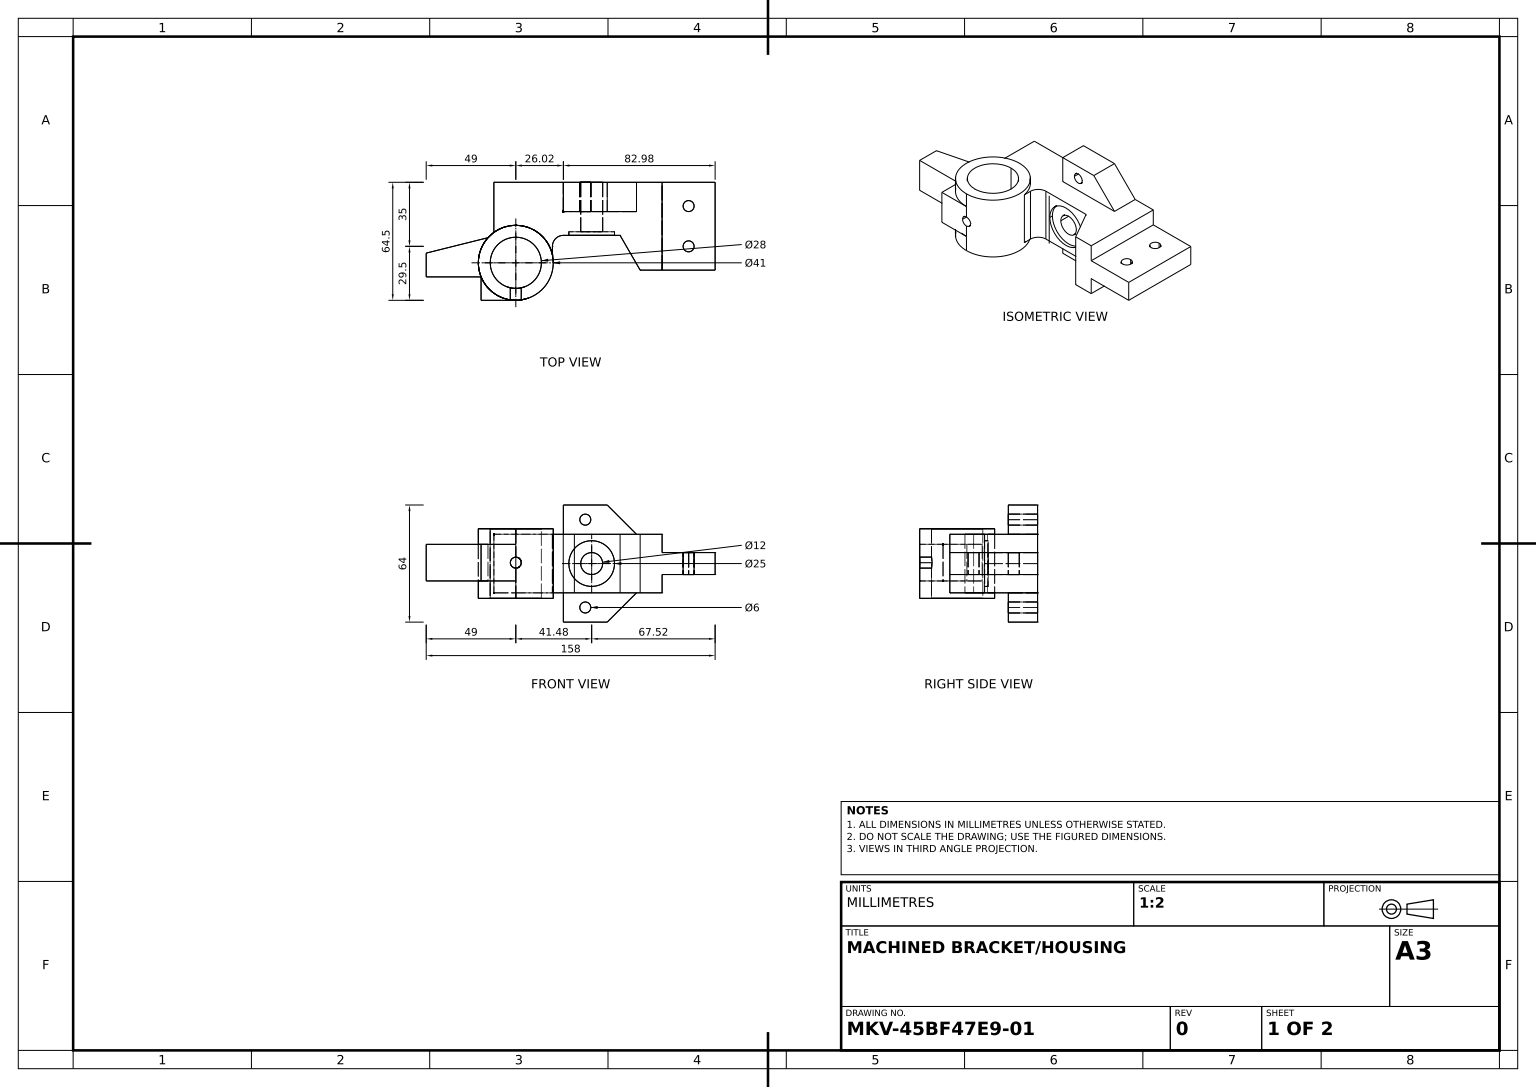
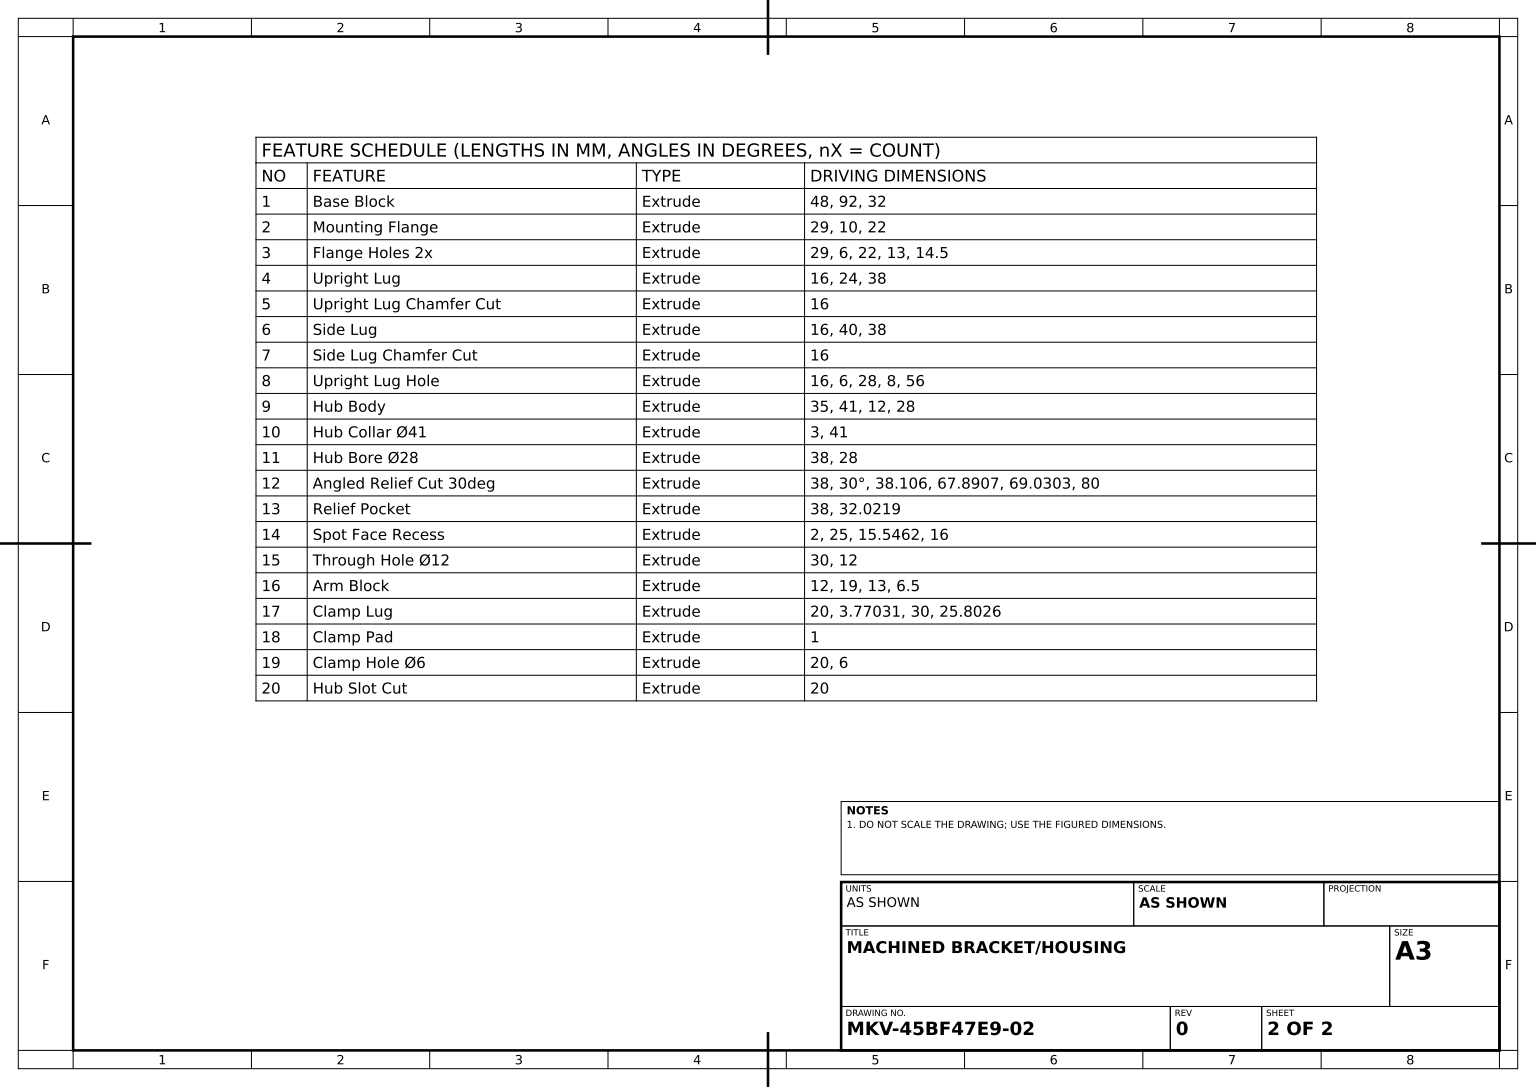
SolidWorks part; units mm, degrees
material "Plain Carbon Steel"
ref_plane "Front Plane" through (0, 0, 0) normal (0, 0, 1) x (1, 0, 0)
ref_plane "Top Plane" through (0, 0, 0) normal (0, 1, 0) x (1, 0, 0)
ref_plane "Right Plane" through (0, 0, 0) normal (1, 0, 0) x (0, 0, -1)
sketch "Base Block Sketch" plane through (0, 0, 0) normal (0, 0, 1) x (1, 0, 0)
  line L0 (0, 0) -> (92, 0)
  line L1 (92, 0) -> (92, 32)
  line L2 (92, 32) -> (0, 32)
  line L3 (0, 32) -> (0, 0)
  dimension "D1" = 92
  dimension "D2" = 32
extrude "Base Block" add sketch "Base Block Sketch" along normal blind 48
sketch "Mounting Flange Sketch" plane through (92, 0, 0) normal (1, 0, 0) x (0, 0, -1)
  line L0 (-48, 22) -> (-48, 10)
  line L1 (-48, 0) -> (-48, 32) construction
  line L2 (-48, 22) -> (0, 22)
  line L3 (0, 0) -> (0, 32) construction
  line L4 (0, 22) -> (0, 10)
  line L5 (0, 10) -> (-48, 10)
  line L6 (-48, 32) -> (0, 32) construction
  dimension "D1" = 10
  dimension "D2" = 22
extrude "Mounting Flange" add sketch "Mounting Flange Sketch" along normal blind 29
sketch "Flange Holes Sketch" plane through (0, 10, 0) normal (0, -1, 0) x (1, 0, 0)
  line L0 (121, 0) -> (92, 0) construction
  line L2 (121, 48) -> (121, 0) construction
  circle A0 centre (106.5, 13) radius 3
  circle A1 centre (106.5, 35) radius 3
  dimension "D1" = 6
  dimension "D2" = 6
  dimension "D3" = 22
  dimension "D4" = 13
  dimension "D5" = 14.5
  dimension "D6" = 14.5
extrude "Flange Holes 2x" cut sketch "Flange Holes Sketch" against normal blind 29
sketch "Upright Lug Sketch" plane through (0, 0, 0) normal (0, -1, 0) x (1, 0, 0)
  line L1 (0, 0) -> (92, 0) construction
  line L2 (38, 0) -> (62, 0)
  line L3 (62, 0) -> (78, 0)
  line L4 (78, 0) -> (78, 16)
  line L5 (78, 16) -> (62, 16)
  line L6 (62, 16) -> (38, 16)
  line L7 (38, 16) -> (38, 0)
  dimension "D1" = 16
  dimension "D2" = 24
  dimension "D3" = 16
  dimension "D4" = 16
  dimension "D5" = 38
extrude "Upright Lug" add sketch "Upright Lug Sketch" along normal blind 16
sketch "Upright Lug Chamfer Sketch" plane through (0, 0, 16) normal (0, 0, 1) x (1, 0, 0)
  line L0 (78, -16) -> (62, -16)
  line L1 (78, -16) -> (38, -16) construction
  line L2 (62, -16) -> (78, 0)
  line L3 (78, 0) -> (78, -16)
extrude "Upright Lug Chamfer Cut" cut sketch "Upright Lug Chamfer Sketch" against normal blind 16
sketch "Side Lug Sketch" plane through (0, 32, 0) normal (0, 1, 0) x (1, 0, 0)
  line L0 (0, -48) -> (0, 0) construction
  line L1 (92, 0) -> (0, 0) construction
  line L2 (38, 0) -> (62, 0)
  line L3 (62, 0) -> (78, 0)
  line L4 (78, 0) -> (78, -16)
  line L5 (78, -16) -> (62, -16)
  line L6 (62, -16) -> (38, -16)
  line L7 (38, -16) -> (38, 0)
  dimension "D1" = 16
  dimension "D2" = 40
  dimension "D3" = 38
extrude "Side Lug" add sketch "Side Lug Sketch" along normal blind 16
sketch "Side Lug Chamfer Sketch" plane through (0, 0, 16) normal (0, 0, 1) x (1, 0, 0)
  line L0 (78, 48) -> (62, 48)
  line L1 (38, 48) -> (78, 48) construction
  line L2 (62, 48) -> (78, 32)
  line L3 (78, 32) -> (78, 48)
extrude "Side Lug Chamfer Cut" cut sketch "Side Lug Chamfer Sketch" against normal blind 16
sketch "Upright Lug Hole Sketch" plane through (0, 0, 16) normal (0, 0, 1) x (1, 0, 0)
  line L0 (62, -16) -> (38, -16) construction
  circle A0 centre (50, 40) radius 3
  circle A1 centre (50, -8) radius 3
  dimension "D1" = 6
  dimension "D2" = 6
  dimension "D3" = 6
  dimension "D4" = 6
  dimension "D5" = 28
  dimension "D6" = 8
  dimension "D7" = 56
extrude "Upright Lug Hole" cut sketch "Upright Lug Hole Sketch" against normal blind 16
sketch "Hub Body Sketch" plane through (0, 0, 0) normal (0, -1, 0) x (1, 0, 0)
  line L0 (0, 0) -> (12, 0)
  line L1 (0, 0) -> (38, 0) construction
  line L2 (0, 48) -> (0, 0) construction
  line L4 (78, 16) -> (38, 16) construction
  circle A0 centre (12, 44) radius 20.5
  line M6 (92, 48) -> (0, 48)
  line M7 (0, 48) -> (0, 0)
  dimension "D1" = 41
  dimension "D2" = 41
  dimension "D3" = 12
  dimension "D4" = 28
extrude "Hub Body" add sketch "Hub Body Sketch" against normal blind 35 contours A0 M6 M7 | A0 M7 M6
sketch "Hub Collar Sketch" plane through (0, 0, 0) normal (0, -1, 0) x (1, 0, 0)
  circle A0 centre (12, 44) radius 20.5
  dimension "D1" = 41
  dimension "D2" = 41
extrude "Hub Collar Ø41" add sketch "Hub Collar Sketch" along normal blind 3
sketch "Hub Bore Sketch" plane through (0, -3, 0) normal (0, -1, 0) x (1, 0, 0)
  circle A0 centre (12, 44) radius 14
  dimension "D1" = 28
  dimension "D2" = 28
extrude "Hub Bore Ø28" cut sketch "Hub Bore Sketch" against normal blind 38
sketch "Angled Relief Sketch" plane through (0, 0, 0) normal (0, -1, 0) x (1, 0, 0)
  line L0 (92, 48) -> (80, 48)
  line L1 (32.106, 48) -> (92, 48) construction
  line L2 (80, 48) -> (69.0303, 29)
  line L3 (0, 27.3792) -> (0, 0) construction
  line L4 (67.8907, 29) -> (69.0303, 29)
  line L6 (92, 48) -> (92, 0) construction
  line L8 (67.8907, 29) -> (38.106, 29)
  line L10 (38.106, 48) -> (80, 48)
  line L11 (38.106, 48) -> (38.106, 29)
  line L12 (38.106, 48) -> (80, 48)
  point P11 (32.106, 48)
  line M11 (92, 48) -> (32.106, 48)
  dimension "D2" = 38.106
  dimension "D1" = 30
  dimension "D3" = 67.8907
  dimension "D4" = 69.0303
  dimension "D5" = 80
extrude "Angled Relief Cut 30deg" cut sketch "Angled Relief Sketch" against normal blind 38 contours L11 L8 L4 L2 M11
sketch "Relief Pocket Sketch" plane through (0, 0, 0) normal (0, -1, 0) x (1, 0, 0)
  line L0 (32.0219, 34.9994) -> (32.106, 48)
  line L1 (0, 27.3792) -> (0, 0) construction
  line L2 (38.106, 29) -> (37.9379, 29)
  line L5 (32.106, 48) -> (38.106, 48)
  line L6 (38.106, 48) -> (38.106, 29)
  arc A0 (32.0219, 34.9994) -> (38.106, 29) centre (38.0219, 34.9994) ccw
  line M3 (38.106, 29) -> (38.106, 48)
  line M4 (38.106, 48) -> (32.106, 48)
  arc M5 (32.106, 48) -> (0, 27.3792) centre (12, 44) cw
  dimension "D1" = 6
  dimension "D2" = 32.0219
extrude "Relief Pocket" cut sketch "Relief Pocket Sketch" against normal blind 38 contours L0 A0 L2 M3 M4 M5
sketch "Spot Face Sketch" plane through (0, 0, 29) normal (0, 0, 1) x (1, 0, 0)
  line L0 (37.9379, 32) -> (37.9379, 0) construction
  line L1 (69.0303, 32) -> (37.9379, 32) construction
  circle A0 centre (53.4841, 16) radius 12.5
  dimension "D1" = 15.5462
  dimension "D2" = 25
  dimension "D3" = 16
extrude "Spot Face Recess" cut sketch "Spot Face Sketch" against normal blind 2
sketch "Through Hole Sketch" plane through (0, 0, 27) normal (0, 0, 1) x (1, 0, 0)
  circle A0 centre (53.4841, 16) radius 6
  dimension "D1" = 12
  dimension "D2" = 12
extrude "Through Hole Ø12" cut sketch "Through Hole Sketch" against normal blind 30
ref_plane "Plane1" through (-8, 0, 0) normal (1, 0, 0) x (0, 0, -1)
ref_plane "Arm Offset Plane" through (12, 0, 0) normal (1, 0, 0) x (0, 0, -1)
sketch "Arm Block Sketch" plane through (12, 0, 0) normal (1, 0, 0) x (0, 0, -1)
  line L1 (-64.5, 35) -> (-64.5, -3) construction
  line L2 (-64.5, 25.5) -> (-51.5, 25.5)
  line L3 (-51.5, 25.5) -> (-51.5, 6.5)
  line L4 (-51.5, 6.5) -> (-64.5, 6.5)
  line L6 (-64.5, 25.5) -> (-64.5, 6.5)
  dimension "D1" = 13
  dimension "D2" = 19
  dimension "D3" = 6.5
extrude "Arm Block" add sketch "Arm Block Sketch" against normal blind 19
sketch "Clamp Lug Sketch" plane through (0, 6.5, 0) normal (0, -1, 0) x (1, 0, 0)
  line L0 (-7, 51.6974) -> (-37, 51.6974)
  line L1 (-37, 51.6974) -> (-37, 38.6974)
  line L2 (-37, 38.6974) -> (-3.2297, 30.2775)
  line L3 (-7, 64.5) -> (-7, 51.6974) construction
  arc A0 (-7, 51.6974) -> (-3.2297, 30.2775) centre (12, 44) ccw
  dimension "D1" = 41
  dimension "D2" = 3.7703
  dimension "D3" = 30
  dimension "D4" = 25.8026
extrude "Clamp Lug" add sketch "Clamp Lug Sketch" against normal blind 20
sketch "Clamp Pad Sketch" plane through (0, 25.5, 0) normal (0, 1, 0) x (1, 0, 0)
  line L0 (-7, -51.6974) -> (-7, -64.5)
  line L1 (-7, -51.6974) -> (-7, -64.5) construction
  line L2 (-7, -64.5) -> (12, -64.5)
  line L3 (-7, -64.5) -> (12, -64.5) construction
  circle A0 centre (12, -44) radius 20.5 construction
  arc A1 (-7, -51.6974) -> (12, -64.5) centre (12, -44) ccw
  dimension "D1" = 41
extrude "Clamp Pad" add sketch "Clamp Pad Sketch" along normal blind 1
sketch "Clamp Hole Sketch" plane through (0, 0, 64.5) normal (0, 0, 1) x (1, 0, 0)
  line L0 (12, 26.5) -> (12, 6.5) construction
  circle A0 centre (12, 16.5) radius 3
  dimension "D1" = 6
  dimension "D2" = 6
extrude "Clamp Hole Ø6" cut sketch "Clamp Hole Sketch" against normal blind 20
sketch "Hub Slot Sketch" plane through (0, 6.5, 0) normal (0, -1, 0) x (1, 0, 0)
  line L0 (12, 51.5) -> (12, 58)
  line L1 (12, 51.5) -> (0.1784, 51.5)
  arc A0 (12, 58) -> (0.1784, 51.5) centre (12, 44) ccw
  dimension "D1" = 28
extrude "Hub Slot Cut" cut sketch "Hub Slot Sketch" against normal blind 20
